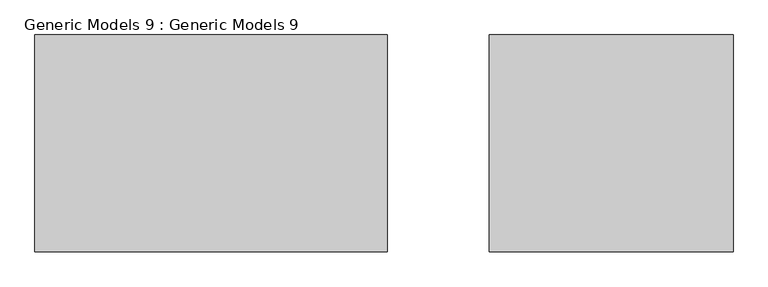
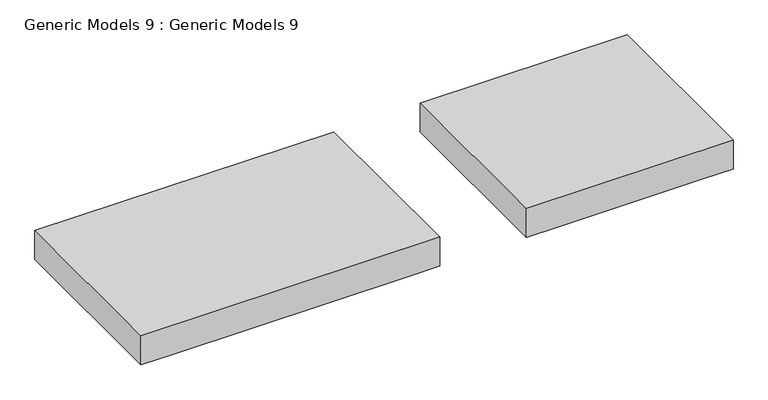
"""IFC4 building model written with IfcOpenShell, lengths in millimetres: proxy geometry, Generic Models 9 : Generic Models 9."""

from ifc_helpers import new_model, si_unit, frame, origin, place, context, project, spatial, polyline, outline, extrude, source, transform, mapped, element, save


def generic_models_9_generic_models_9_114c8f56(model_context):
    return source(origin(), model_context, "Body", "SweptSolid", [
        extrude(outline(polyline([(2190.75, -30014.9645004), (2190.75, -29862.5645004), (2190.75, -28681.4645004), (2190.75, -28529.0645004), (2343.15, -28529.0645004), (2343.15, -30014.9645004), (2190.75, -30014.9645004)])), frame((0.0, 19682.7756148, 0.0), z_axis=(0.0, 1.0, 0.0), x_axis=(0.0, 0.0, 1.0)), (0.0, 0.0, 1.0), 914.4),
        extrude(outline(polyline([(2190.75, -28097.2645004), (2190.75, -27944.8645004), (2190.75, -27220.9645004), (2190.75, -27068.5645004), (2343.15, -27068.5645004), (2343.15, -28097.2645004), (2190.75, -28097.2645004)])), frame((0.0, 19682.7756148, 0.0), z_axis=(0.0, 1.0, 0.0), x_axis=(0.0, 0.0, 1.0)), (0.0, 0.0, 1.0), 914.4),
    ])


if __name__ == "__main__":
    model = new_model("IFC4")
    model_context = context("Model", 3, world=origin())
    ifc_project = project(units=[si_unit("LENGTHUNIT", "METRE", prefix="MILLI")], contexts=[model_context])
    site = spatial("IfcSite", under=ifc_project)
    building = spatial("IfcBuilding", under=site)
    placement = place(None, origin())
    generic_models_9_generic_models_9_shape = generic_models_9_generic_models_9_114c8f56(model_context)
    element("IfcBuildingElementProxy", 1, Name="Generic Models 9 : Generic Models 9", ObjectType="Generic Models 9 : Generic Models 9", at=placement, inside=building, context=model_context, shape_type="MappedRepresentation", body=[
        mapped(generic_models_9_generic_models_9_shape, transform((0.0, 0.0, 0.0), x_axis=(1.0, 0.0, 0.0), y_axis=(0.0, 1.0, 0.0), z_axis=(0.0, 0.0, 1.0))),
    ])
    save(model, "model.ifc")
